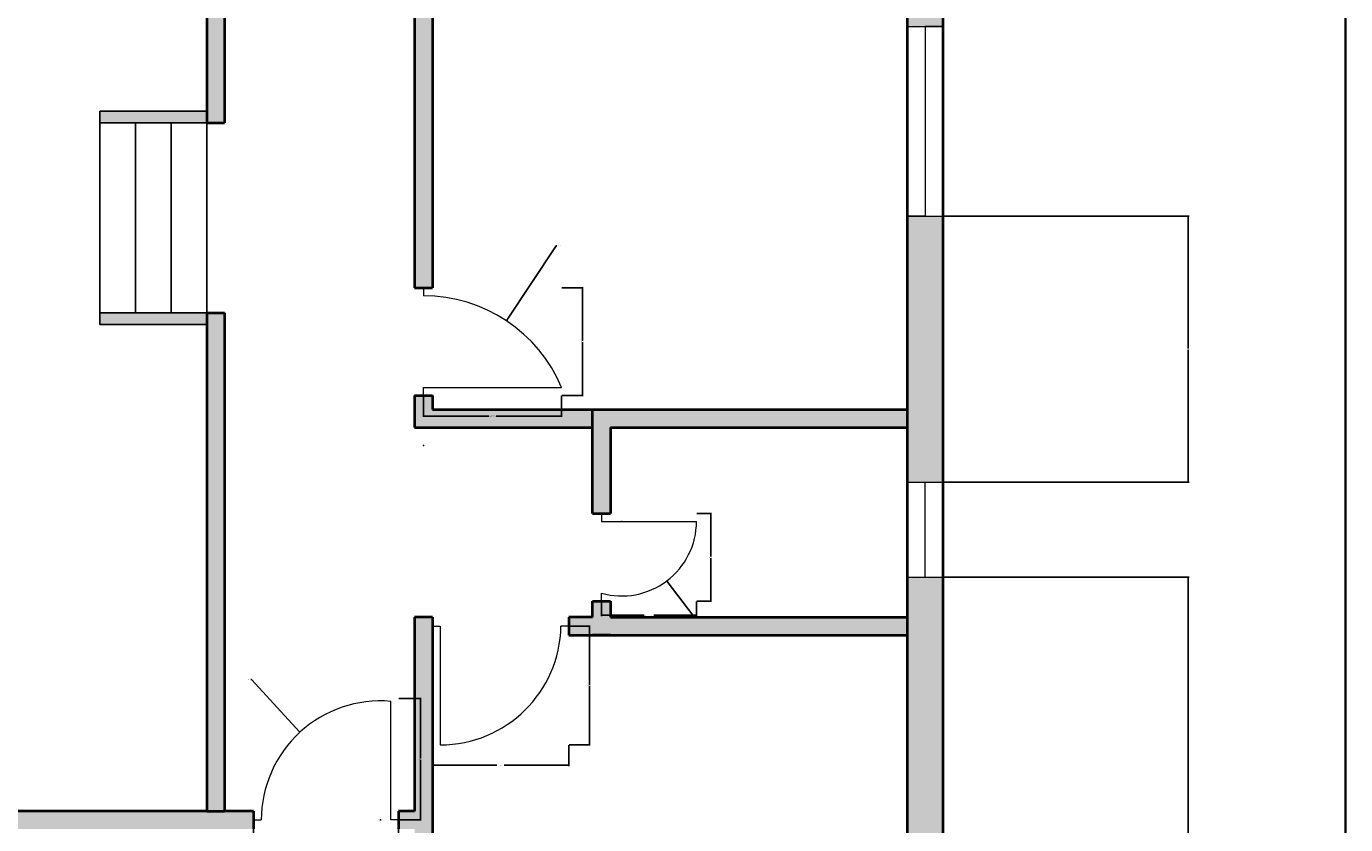
# Model space of a CAD drawing. Units: inches. Extents: x 1441 to 2460, y 1648 to 2683.
# Tile 32 of 35: x 2127 to 2460, y 1922 to 2124. Entities that reach past the tile are written whole.
import ezdxf

# ---------------------------------------------------------------- set-up
doc = ezdxf.new("R2010")
doc.units = ezdxf.units.IN
for name, color, linetype, lineweight in [('A-ANNO-DIMS', 2, 'Continuous', 18), ('A-ANNO-TTLB', 7, 'Continuous', 35), ('A-DOOR', 3, 'Continuous', 20), ('A-FLOR-STRS', 7, 'Continuous', 25), ('A-GLAZ', 4, 'Continuous', 18), ('A-WALL', 7, 'Continuous', 40)]:
    doc.layers.add(name, color=color, linetype=linetype, lineweight=lineweight)
doc.layers.add('A-WALL-PATT', color=251, linetype='Continuous', lineweight=13, true_color=0x636466)
doc.styles.get("Standard").update_dxf_attribs({"font": 'arial.ttf'})
doc.dimstyles.get("Standard").update_dxf_attribs({"dimtxt": 0.18, "dimasz": 0.18, "dimexe": 0.18, "dimexo": 0.0625, "dimgap": 0.09, "dimtad": 0, "dimtih": 1, "dimtoh": 1, "dimdec": 4, "dimzin": 0, "dimdsep": 46, "dimtxsty": 'Standard', "dimcen": 0.09, "dimadec": 0, "dimazin": 0, "dimtfac": 1, "dimtdec": 4, "dimtofl": 0, "dimtmove": 0, "dimatfit": 3, "dimfxl": 1, "dimtolj": 1, "dimtzin": 0, "dimarcsym": 0})

# ---------------------------------------------------------------- blocks, each defined once
blk = doc.blocks.new('DOOR-BED2-30')
for p, q in [((0, 27.22), (0, 25.22)), ((0, 0), (0, 2)), ((0, 2), (4.91, 2)), ((4.91, 2), (34.91, 2))]:
    blk.add_line(p, q)
blk.add_arc((0, -12.65), 37.87, 22.7676, 90)
blk = doc.blocks.new('DOOR-WC-SOUTH-24')
for p, q in [((0, 22.15), (0, 20.15)), ((0, 20.15), (24, 20.15)), ((0, 0), (0, 2))]:
    blk.add_line(p, q)
blk.add_arc((5.13, 20.15), 18.86, 254.1904, 0)
blk = doc.blocks.new('DOOR-BED3-30')
for p, q in [((0, 30.01), (2, 30.01)), ((2, 30.01), (2, 0.01)), ((34.49, 30.01), (32.49, 30.01))]:
    blk.add_line(p, q)
blk.add_arc((2, 30.51), 30.5, 270, 359.0598)
blk = doc.blocks.new('DOOR-ENTRY-INNER')
for p, q in [((34.71, 24.01), (34.71, 30.01)), ((34.71, 0.01), (34.71, 24.01)), ((0, 0.01), (2, 0.01)), ((36.71, 0.01), (34.71, 0.01))]:
    blk.add_line(p, q)
blk.add_arc((32.11, 0.01), 30.11, 85.0485, 180)
blk = doc.blocks.new('WIN-48-SASH')
for p, q in [((9, 48), (4.5, 48)), ((4.5, 48), (4.5, 0)), ((4.5, 0), (0, 0))]:
    blk.add_line(p, q)
blk = doc.blocks.new('WIN-24-SASH')
for p, q in [((9, 24), (4.5, 24)), ((4.5, 24), (4.5, 0)), ((4.5, 0), (0, 0))]:
    blk.add_line(p, q)
blk = doc.blocks.new('*D48')
at = {"layer": 'A-ANNO-DIMS', "color": 0, "lineweight": -2, "transparency": 16777216}
for p, q in [((2227.15, 2030.73), (2227.15, 2025.37)), ((2262.07, 2030.73), (2262.07, 2025.37)), ((2227.33, 2025.55), (2243.68, 2025.55)), ((2261.89, 2025.55), (2245.54, 2025.55))]:
    blk.add_line(p, q, dxfattribs=at)
at = {"layer": 'A-ANNO-DIMS', "color": 0, "transparency": 16777216}
for points in [[(2227.33, 2025.58), (2227.33, 2025.52), (2227.15, 2025.55)], [(2261.89, 2025.58), (2261.89, 2025.52), (2262.07, 2025.55)]]:
    blk.add_solid(points, dxfattribs=at)
at = {"layer": 'Defpoints', "color": 0, "transparency": 16777216}
for p in [(2227.15, 2030.79), (2262.07, 2030.79), (2262.07, 2025.55)]:
    blk.add_point(p, dxfattribs=at)
at = {"layer": 'A-ANNO-DIMS', "color": 0, "transparency": 16777216, "insert": (2244.61, 2025.55), "char_height": 0.18, "attachment_point": 5}
blk.add_mtext('\\A1;B2 DR 35 TYP.', dxfattribs=at)
blk = doc.blocks.new('*D49')
at = {"layer": 'A-ANNO-DIMS', "color": 0, "lineweight": -2, "transparency": 16777216}
for p, q in [((2262.13, 2058.01), (2267.49, 2058.01)), ((2267.31, 2057.83), (2267.31, 2044.58)), ((2267.31, 2030.97), (2267.31, 2044.22)), ((2262.13, 2030.79), (2267.49, 2030.79))]:
    blk.add_line(p, q, dxfattribs=at)
at = {"layer": 'A-ANNO-DIMS', "color": 0, "transparency": 16777216}
for points in [[(2267.28, 2057.83), (2267.34, 2057.83), (2267.31, 2058.01)], [(2267.28, 2030.97), (2267.34, 2030.97), (2267.31, 2030.79)]]:
    blk.add_solid(points, dxfattribs=at)
at = {"layer": 'Defpoints', "color": 0, "transparency": 16777216}
for p in [(2262.07, 2058.01), (2267.31, 2058.01), (2262.07, 2030.79)]:
    blk.add_point(p, dxfattribs=at)
at = {"layer": 'A-ANNO-DIMS', "color": 0, "transparency": 16777216, "insert": (2267.31, 2044.4), "char_height": 0.18, "attachment_point": 5}
blk.add_mtext('\\A1;27 TYP.', dxfattribs=at)
blk = doc.blocks.new('*D50')
at = {"layer": 'A-ANNO-DIMS', "color": 0, "lineweight": -2, "transparency": 16777216}
for p, q in [((2272.15, 1978.73), (2272.15, 1975.02)), ((2296.15, 1978.73), (2296.15, 1975.02)), ((2272.33, 1975.2), (2282.96, 1975.2)), ((2295.97, 1975.2), (2285.34, 1975.2))]:
    blk.add_line(p, q, dxfattribs=at)
at = {"layer": 'A-ANNO-DIMS', "color": 0, "transparency": 16777216}
for points in [[(2272.33, 1975.23), (2272.33, 1975.17), (2272.15, 1975.2)], [(2295.97, 1975.23), (2295.97, 1975.17), (2296.15, 1975.2)]]:
    blk.add_solid(points, dxfattribs=at)
at = {"layer": 'Defpoints', "color": 0, "transparency": 16777216}
for p in [(2272.15, 1978.8), (2296.15, 1978.8), (2296.15, 1975.2)]:
    blk.add_point(p, dxfattribs=at)
at = {"layer": 'A-ANNO-DIMS', "color": 0, "transparency": 16777216, "insert": (2284.15, 1975.2), "char_height": 0.18, "attachment_point": 5}
blk.add_mtext('\\A1;WC DOOR 24 TYP.', dxfattribs=at)
blk = doc.blocks.new('*D51')
at = {"layer": 'A-ANNO-DIMS', "color": 0, "lineweight": -2, "transparency": 16777216}
for p, q in [((2296.21, 2000.95), (2299.93, 2000.95)), ((2299.75, 2000.77), (2299.75, 1990.05)), ((2299.75, 1978.98), (2299.75, 1989.69)), ((2296.21, 1978.8), (2299.93, 1978.8))]:
    blk.add_line(p, q, dxfattribs=at)
at = {"layer": 'A-ANNO-DIMS', "color": 0, "transparency": 16777216}
for points in [[(2299.72, 2000.77), (2299.78, 2000.77), (2299.75, 2000.95)], [(2299.72, 1978.98), (2299.78, 1978.98), (2299.75, 1978.8)]]:
    blk.add_solid(points, dxfattribs=at)
at = {"layer": 'Defpoints', "color": 0, "transparency": 16777216}
for p in [(2296.15, 2000.95), (2299.75, 2000.95), (2296.15, 1978.8)]:
    blk.add_point(p, dxfattribs=at)
at = {"layer": 'A-ANNO-DIMS', "color": 0, "transparency": 16777216, "insert": (2299.75, 1989.87), "char_height": 0.18, "attachment_point": 5}
blk.add_mtext('\\A1;22 TYP.', dxfattribs=at)
blk = doc.blocks.new('*D52')
at = {"layer": 'A-ANNO-DIMS', "color": 0, "lineweight": -2, "transparency": 16777216}
for p, q in [((2229.4, 1942.38), (2229.4, 1937.09)), ((2263.9, 1942.38), (2263.9, 1937.09)), ((2229.58, 1937.27), (2245.72, 1937.27)), ((2263.72, 1937.27), (2247.58, 1937.27))]:
    blk.add_line(p, q, dxfattribs=at)
at = {"layer": 'A-ANNO-DIMS', "color": 0, "transparency": 16777216}
for points in [[(2229.58, 1937.3), (2229.58, 1937.24), (2229.4, 1937.27)], [(2263.72, 1937.3), (2263.72, 1937.24), (2263.9, 1937.27)]]:
    blk.add_solid(points, dxfattribs=at)
at = {"layer": 'Defpoints', "color": 0, "transparency": 16777216}
for p in [(2229.4, 1942.45), (2263.9, 1942.45), (2263.9, 1937.27)]:
    blk.add_point(p, dxfattribs=at)
at = {"layer": 'A-ANNO-DIMS', "color": 0, "transparency": 16777216, "insert": (2246.65, 1937.27), "char_height": 0.18, "attachment_point": 5}
blk.add_mtext('\\A1;B3 DR 34 TYP.', dxfattribs=at)
blk = doc.blocks.new('*D53')
at = {"layer": 'A-ANNO-DIMS', "color": 0, "lineweight": -2, "transparency": 16777216}
for p, q in [((2263.96, 1972.45), (2269.25, 1972.45)), ((2269.07, 1972.27), (2269.07, 1957.63)), ((2269.07, 1942.63), (2269.07, 1957.26)), ((2263.96, 1942.45), (2269.25, 1942.45))]:
    blk.add_line(p, q, dxfattribs=at)
at = {"layer": 'A-ANNO-DIMS', "color": 0, "transparency": 16777216}
for points in [[(2269.04, 1972.27), (2269.1, 1972.27), (2269.07, 1972.45)], [(2269.04, 1942.63), (2269.1, 1942.63), (2269.07, 1942.45)]]:
    blk.add_solid(points, dxfattribs=at)
at = {"layer": 'Defpoints', "color": 0, "transparency": 16777216}
for p in [(2263.9, 1972.45), (2269.07, 1972.45), (2263.9, 1942.45)]:
    blk.add_point(p, dxfattribs=at)
at = {"layer": 'A-ANNO-DIMS', "color": 0, "transparency": 16777216, "insert": (2269.07, 1957.45), "char_height": 0.18, "attachment_point": 5}
blk.add_mtext('\\A1;30 TYP.', dxfattribs=at)
blk = doc.blocks.new('*D56')
at = {"layer": 'A-ANNO-DIMS', "color": 0, "lineweight": -2, "transparency": 16777216}
for p, q in [((2184.17, 1923.38), (2184.17, 1917.76)), ((2220.88, 1923.38), (2220.88, 1917.76)), ((2184.35, 1917.94), (2201.59, 1917.94)), ((2220.7, 1917.94), (2203.46, 1917.94))]:
    blk.add_line(p, q, dxfattribs=at)
at = {"layer": 'A-ANNO-DIMS', "color": 0, "transparency": 16777216}
for points in [[(2184.35, 1917.97), (2184.35, 1917.91), (2184.17, 1917.94)], [(2220.7, 1917.97), (2220.7, 1917.91), (2220.88, 1917.94)]]:
    blk.add_solid(points, dxfattribs=at)
at = {"layer": 'Defpoints', "color": 0, "transparency": 16777216}
for p in [(2184.17, 1923.45), (2220.88, 1923.45), (2220.88, 1917.94)]:
    blk.add_point(p, dxfattribs=at)
at = {"layer": 'A-ANNO-DIMS', "color": 0, "transparency": 16777216, "insert": (2202.52, 1917.94), "char_height": 0.18, "attachment_point": 5}
blk.add_mtext('\\A1;DOOR 37 TYP.', dxfattribs=at)
blk = doc.blocks.new('*D57')
at = {"layer": 'A-ANNO-DIMS', "color": 0, "lineweight": -2, "transparency": 16777216}
for p, q in [((2220.94, 1954.17), (2226.56, 1954.17)), ((2226.38, 1953.99), (2226.38, 1938.99)), ((2226.38, 1923.63), (2226.38, 1938.63)), ((2220.94, 1923.45), (2226.56, 1923.45))]:
    blk.add_line(p, q, dxfattribs=at)
at = {"layer": 'A-ANNO-DIMS', "color": 0, "transparency": 16777216}
for points in [[(2226.35, 1953.99), (2226.41, 1953.99), (2226.38, 1954.17)], [(2226.35, 1923.63), (2226.41, 1923.63), (2226.38, 1923.45)]]:
    blk.add_solid(points, dxfattribs=at)
at = {"layer": 'Defpoints', "color": 0, "transparency": 16777216}
for p in [(2220.88, 1954.17), (2226.38, 1954.17), (2220.88, 1923.45)]:
    blk.add_point(p, dxfattribs=at)
at = {"layer": 'A-ANNO-DIMS', "color": 0, "transparency": 16777216, "insert": (2226.38, 1938.81), "char_height": 0.18, "attachment_point": 5}
blk.add_mtext('\\A1;31 TYP.', dxfattribs=at)
blk = doc.blocks.new('*D81')
at = {"layer": 'A-ANNO-DIMS', "color": 0, "lineweight": -2, "transparency": 16777216}
for p, q in [((2037.84, 2298.7), (1976.42, 2298.7)), ((1976.6, 2298.52), (1976.6, 2055.94)), ((1976.6, 1813), (1976.6, 2055.57)), ((2154.24, 1812.82), (1976.42, 1812.82))]:
    blk.add_line(p, q, dxfattribs=at)
at = {"layer": 'A-ANNO-DIMS', "color": 0, "transparency": 16777216}
for points in [[(1976.57, 2298.52), (1976.63, 2298.52), (1976.6, 2298.7)], [(1976.57, 1813), (1976.63, 1813), (1976.6, 1812.82)]]:
    blk.add_solid(points, dxfattribs=at)
at = {"layer": 'Defpoints', "color": 0, "transparency": 16777216}
for p in [(1976.6, 2298.7), (2037.9, 2298.7), (2154.3, 1812.82)]:
    blk.add_point(p, dxfattribs=at)
at = {"layer": 'A-ANNO-DIMS', "color": 0, "transparency": 16777216, "insert": (1976.6, 2055.76), "char_height": 0.18, "attachment_point": 5}
blk.add_mtext('\\A1;485.9', dxfattribs=at)
blk = doc.blocks.new('*D86')
at = {"layer": 'A-ANNO-DIMS', "color": 0, "lineweight": -2, "transparency": 16777216}
for p, q in [((2358.46, 1984.83), (2420.62, 1984.83)), ((2420.44, 1984.65), (2420.44, 1909.69)), ((2420.44, 1834.38), (2420.44, 1909.33)), ((2358.46, 1834.2), (2420.62, 1834.2))]:
    blk.add_line(p, q, dxfattribs=at)
at = {"layer": 'A-ANNO-DIMS', "color": 0, "transparency": 16777216}
for points in [[(2420.41, 1984.65), (2420.47, 1984.65), (2420.44, 1984.83)], [(2420.41, 1834.38), (2420.47, 1834.38), (2420.44, 1834.2)]]:
    blk.add_solid(points, dxfattribs=at)
at = {"layer": 'Defpoints', "color": 0, "transparency": 16777216}
for p in [(2358.4, 1984.83), (2420.44, 1984.83), (2358.4, 1834.2)]:
    blk.add_point(p, dxfattribs=at)
at = {"layer": 'A-ANNO-DIMS', "color": 0, "transparency": 16777216, "insert": (2420.44, 1909.51), "char_height": 0.18, "attachment_point": 5}
blk.add_mtext('\\A1;150.64', dxfattribs=at)
blk = doc.blocks.new('*D87')
at = {"layer": 'A-ANNO-DIMS', "color": 0, "lineweight": -2, "transparency": 16777216}
for p, q in [((2358.46, 2076.11), (2420.62, 2076.11)), ((2420.44, 2075.93), (2420.44, 2042.65)), ((2420.44, 2009.01), (2420.44, 2042.29)), ((2358.46, 2008.83), (2420.62, 2008.83))]:
    blk.add_line(p, q, dxfattribs=at)
at = {"layer": 'A-ANNO-DIMS', "color": 0, "transparency": 16777216}
for points in [[(2420.41, 2075.93), (2420.47, 2075.93), (2420.44, 2076.11)], [(2420.41, 2009.01), (2420.47, 2009.01), (2420.44, 2008.83)]]:
    blk.add_solid(points, dxfattribs=at)
at = {"layer": 'Defpoints', "color": 0, "transparency": 16777216}
for p in [(2358.4, 2076.11), (2420.44, 2076.11), (2358.4, 2008.83)]:
    blk.add_point(p, dxfattribs=at)
at = {"layer": 'A-ANNO-DIMS', "color": 0, "transparency": 16777216, "insert": (2420.44, 2042.47), "char_height": 0.18, "attachment_point": 5}
blk.add_mtext('\\A1;67.28', dxfattribs=at)
blk = doc.blocks.new('*D129')
at = {"layer": 'A-ANNO-DIMS', "color": 0, "lineweight": -2, "transparency": 16777216}
for p, q in [((2260.7, 2068.59), (2248.22, 2049.82)), ((2260.88, 2068.59), (2260.7, 2068.59)), ((2227.06, 2018.14), (2227.24, 2018.14)), ((2227.15, 2018.05), (2227.15, 2018.23))]:
    blk.add_line(p, q, dxfattribs=at)
at = {"layer": 'A-ANNO-DIMS', "color": 0, "transparency": 16777216}
blk.add_solid([(2248.19, 2049.84), (2248.24, 2049.81), (2248.12, 2049.67)], dxfattribs=at)
at = {"layer": 'Defpoints', "color": 0, "transparency": 16777216}
for p in [(2248.12, 2049.67), (2227.15, 2018.14)]:
    blk.add_point(p, dxfattribs=at)
at = {"layer": 'A-ANNO-DIMS', "color": 0, "transparency": 16777216, "insert": (2261.36, 2068.59), "char_height": 0.18, "attachment_point": 5}
blk.add_mtext('\\A1;R37.87', dxfattribs=at)
blk = doc.blocks.new('*D132')
at = {"layer": 'A-ANNO-DIMS', "color": 0, "lineweight": -2, "transparency": 16777216}
for p, q in [((2183.53, 1958.95), (2183.71, 1958.95)), ((2183.71, 1958.95), (2195.8, 1945.77)), ((2216.19, 1923.45), (2216.37, 1923.45)), ((2216.28, 1923.36), (2216.28, 1923.54))]:
    blk.add_line(p, q, dxfattribs=at)
at = {"layer": 'A-ANNO-DIMS', "color": 0, "transparency": 16777216}
blk.add_solid([(2195.83, 1945.79), (2195.78, 1945.75), (2195.93, 1945.64)], dxfattribs=at)
at = {"layer": 'Defpoints', "color": 0, "transparency": 16777216}
for p in [(2195.93, 1945.64), (2216.28, 1923.45)]:
    blk.add_point(p, dxfattribs=at)
at = {"layer": 'A-ANNO-DIMS', "color": 0, "transparency": 16777216, "insert": (2183.07, 1958.95), "char_height": 0.18, "attachment_point": 5}
blk.add_mtext('\\A1;R30.11', dxfattribs=at)
blk = doc.blocks.new('*D135')
at = {"layer": 'A-ANNO-DIMS', "color": 0, "lineweight": -2, "transparency": 16777216}
for p, q in [((2277.2, 1998.95), (2277.38, 1998.95)), ((2277.29, 1998.86), (2277.29, 1999.04)), ((2295.49, 1974.87), (2288.77, 1983.76)), ((2295.67, 1974.87), (2295.49, 1974.87))]:
    blk.add_line(p, q, dxfattribs=at)
at = {"layer": 'A-ANNO-DIMS', "color": 0, "transparency": 16777216}
blk.add_solid([(2288.8, 1983.78), (2288.75, 1983.74), (2288.67, 1983.9)], dxfattribs=at)
at = {"layer": 'Defpoints', "color": 0, "transparency": 16777216}
for p in [(2277.29, 1998.95), (2288.67, 1983.9)]:
    blk.add_point(p, dxfattribs=at)
at = {"layer": 'A-ANNO-DIMS', "color": 0, "transparency": 16777216, "insert": (2296.15, 1974.87), "char_height": 0.18, "attachment_point": 5}
blk.add_mtext('\\A1;R18.86', dxfattribs=at)

msp = doc.modelspace()

# ---------------------------------------------------------------- hatches: boundary and pattern name
at = {"layer": 'A-WALL-PATT'}
h = msp.add_hatch(color=256, dxfattribs=at)
h.dxf.hatch_style = 1
h.paths.add_polyline_path([(2096.524, 2298.6952), (2037.9015, 2298.6952), (2037.9015, 2246.9605), (2046.9015, 2246.9605), (2046.9015, 2289.6952), (2096.524, 2289.6952), (2096.524, 2294.1952)])
h.paths.add_polyline_path([(2144.5933, 2298.6952), (2120.524, 2298.6952), (2120.524, 2289.6952), (2144.5933, 2289.6952), (2144.5933, 2294.1952)])
h.paths.add_polyline_path([(2136.4015, 2289.6952), (2131.9015, 2289.6952), (2131.9015, 2233.0622), (2136.4015, 2233.0622)])
h.paths.add_polyline_path([(2184.8877, 2294.3362), (2184.8877, 2295.2788), (2184.8877, 2298.6952), (2168.5933, 2298.6952), (2168.5933, 2289.6952), (2184.8877, 2289.6952)])
h.paths.add_polyline_path([(2176.9015, 2289.6952), (2172.4015, 2289.6952), (2172.4015, 2199.6952), (2176.9015, 2199.6952)])
h.paths.add_polyline_path([(2229.4015, 2204.637), (2224.9015, 2204.637), (2224.9015, 2199.6952), (2136.4015, 2199.6952), (2136.4015, 2204.637), (2131.9015, 2204.637), (2131.9015, 2195.1952), (2229.4015, 2195.1952)])
h.paths.add_polyline_path([(2229.4015, 2289.6952), (2224.9015, 2289.6952), (2224.9015, 2233.0622), (2229.4015, 2233.0622)])
h.paths.add_polyline_path([(2358.4015, 2298.6952), (2208.8877, 2298.6952), (2208.8877, 2289.6952), (2349.4015, 2289.6952), (2349.4015, 2250.8051), (2358.4015, 2250.8051)])
h.paths.add_polyline_path([(2358.4015, 2202.8051), (2349.4015, 2202.8051), (2349.4015, 2157.6952), (2216.9636, 2157.6952), (2216.9636, 2153.1952), (2224.9015, 2153.1952), (2224.9015, 2058.005), (2229.4015, 2058.005), (2229.4015, 2153.1952), (2349.4015, 2153.1952), (2349.4015, 2124.108), (2358.4015, 2124.108)])
h.paths.add_polyline_path([(2358.4015, 1984.8305), (2349.4015, 1984.8305), (2349.4015, 1834.1952), (2358.4015, 1834.1952)])
h.paths.add_polyline_path([(2358.4015, 2076.108), (2349.4015, 2076.108), (2349.4015, 2008.8305), (2358.4015, 2008.8305)])
h.paths.add_polyline_path([(2349.4015, 2027.1952), (2269.9015, 2027.1952), (2269.9015, 2000.9452), (2274.4015, 2000.9452), (2274.4015, 2022.6952), (2349.4015, 2022.6952)])
h.paths.add_polyline_path([(2269.9015, 2027.1952), (2229.4015, 2027.1952), (2229.4015, 2030.7912), (2224.9015, 2030.7912), (2224.9015, 2022.6952), (2269.9015, 2022.6952)])
h.paths.add_polyline_path([(2349.4015, 1974.6952), (2274.4015, 1974.6952), (2274.4015, 1978.7973), (2269.9015, 1978.7973), (2269.9015, 1974.6952), (2263.8979, 1974.6952), (2263.8979, 1970.1952), (2269.9015, 1970.1952), (2274.4015, 1970.1952), (2349.4015, 1970.1952)])
h.paths.add_polyline_path([(2229.4015, 1974.6952), (2224.9015, 1974.6952), (2224.9015, 1925.6952), (2220.8772, 1925.6952), (2220.8772, 1921.1952), (2229.4015, 1921.1952)])
h.paths.add_polyline_path([(2229.4015, 1921.1952), (2224.9015, 1921.1952), (2224.9015, 1843.1952), (2229.4015, 1843.1952)])
h.paths.add_polyline_path([(2268.1291, 1838.6952), (2268.1291, 1843.1952), (2229.4015, 1843.1952), (2220.91, 1843.1952), (2220.91, 1834.1952), (2227.1771, 1834.1952), (2268.1291, 1834.1952)])
h.paths.add_polyline_path([(2349.4015, 1843.1952), (2328.1291, 1843.1952), (2328.1291, 1834.1952), (2349.4015, 1834.1952)])
h.paths.add_polyline_path([(2046.9015, 1857.7914), (2037.9015, 1857.7914), (2037.9015, 1834.1952), (2164.019, 1834.1952), (2164.019, 1838.6952), (2164.019, 1843.1952), (2046.9015, 1843.1952)])
h.paths.add_polyline_path([(2046.9015, 1959.2399), (2042.4015, 1959.2399), (2037.9015, 1959.2399), (2037.9015, 1905.7914), (2046.9015, 1905.7914), (2046.9015, 1921.1952), (2172.4015, 1921.1952), (2176.9015, 1921.1952), (2184.1657, 1921.1952), (2184.1657, 1925.6952), (2176.9015, 1925.6952), (2172.4015, 1925.6952), (2046.9015, 1925.6952)])
h.paths.add_polyline_path([(2046.9015, 2106.6907), (2037.9015, 2106.6907), (2037.9015, 2019.2399), (2046.9015, 2019.2399)])
h.paths.add_polyline_path([(2176.9015, 2051.6952), (2172.4015, 2051.6952), (2172.4015, 2048.6952), (2172.4015, 1925.6952), (2176.9015, 1925.6952)])
h.paths.add_polyline_path([(2172.4015, 2051.6952), (2145.4015, 2051.6952), (2145.4015, 2048.6952), (2172.4015, 2048.6952)])
h.paths.add_polyline_path([(2172.4015, 2102.6952), (2145.4015, 2102.6952), (2145.4015, 2099.6952), (2154.4015, 2099.6952), (2172.4015, 2099.6952)])
h.paths.add_polyline_path([(2176.9015, 2153.1952), (2179.5767, 2153.1952), (2179.5767, 2157.6952), (2176.9015, 2157.6952), (2176.9015, 2195.1952), (2172.4015, 2195.1952), (2172.4015, 2099.6952), (2176.9015, 2099.6952)])
h.paths.add_polyline_path([(2046.9015, 2198.9605), (2037.9015, 2198.9605), (2037.9015, 2166.6907), (2046.9015, 2166.6907)])

# ---------------------------------------------------------------- linework, layer by layer
at = {"layer": 'A-ANNO-TTLB'}
msp.add_lwpolyline([(1440.5107, 2682.6413), (2460.193, 2682.6413), (2460.193, 1648.08), (1440.5107, 1648.08)], close=True, dxfattribs=at)
at = {"layer": 'A-FLOR-STRS'}
for p, q in [((2172.4015, 2102.6952), (2145.4015, 2102.6952)), ((2145.4015, 2048.6952), (2145.4015, 2102.6952)), ((2172.4015, 2099.6952), (2172.4015, 2102.6952)), ((2172.4015, 2102.6952), (2172.4015, 2099.6952)), ((2172.4015, 2099.6952), (2145.4015, 2099.6952)), ((2154.4015, 2099.6952), (2145.4015, 2099.6952)), ((2145.4015, 2099.6952), (2145.4015, 2048.6952)), ((2154.4015, 2051.6952), (2154.4015, 2099.6952)), ((2172.4015, 2099.6952), (2163.4015, 2099.6952)), ((2163.4015, 2099.6952), (2163.4015, 2051.6952)), ((2172.4015, 2051.6952), (2172.4015, 2099.6952)), ((2172.4015, 2051.6952), (2145.4015, 2051.6952)), ((2163.4015, 2051.6952), (2154.4015, 2051.6952)), ((2172.4015, 2048.6952), (2172.4015, 2051.6952)), ((2172.4015, 2048.6952), (2172.4015, 2051.6952)), ((2172.4015, 2048.6952), (2145.4015, 2048.6952))]:
    msp.add_line(p, q, dxfattribs=at)
at = {"layer": 'A-GLAZ'}
for p, q in [((2349.4015, 2124.108), (2358.4015, 2124.108)), ((2349.4015, 2076.108), (2358.4015, 2076.108)), ((2349.4015, 2008.8305), (2358.4015, 2008.8305)), ((2349.4015, 1984.8305), (2358.4015, 1984.8305))]:
    msp.add_line(p, q, dxfattribs=at)
at = {"layer": 'A-WALL'}
for p, q in [((2358.4015, 2298.6952), (2358.4015, 1834.1952)), ((2172.4015, 2195.1952), (2172.4015, 2099.6952)), ((2176.9015, 2153.1952), (2176.9015, 2099.6952)), ((2224.9015, 2153.1952), (2224.9015, 2058.005)), ((2229.4015, 2153.1952), (2229.4015, 2058.005)), ((2349.4015, 2153.1952), (2349.4015, 1834.1952)), ((2172.4015, 2099.6952), (2176.9015, 2099.6952)), ((2224.9015, 2058.005), (2229.4015, 2058.005)), ((2172.4015, 2051.6952), (2172.4015, 1925.6952)), ((2172.4015, 2051.6952), (2176.9015, 2051.6952)), ((2176.9015, 2051.6952), (2176.9015, 1925.6952)), ((2224.9015, 2030.7912), (2224.9015, 2022.6952)), ((2224.9015, 2030.7912), (2229.4015, 2030.7912)), ((2229.4015, 2030.7912), (2229.4015, 2027.1952)), ((2229.4015, 2027.1952), (2349.4015, 2027.1952)), ((2269.9015, 2000.9452), (2269.9015, 2027.1952)), ((2224.9015, 2022.6952), (2269.9015, 2022.6952)), ((2274.4015, 2022.6952), (2274.4015, 2000.9452)), ((2274.4015, 2022.6952), (2349.4015, 2022.6952)), ((2269.9015, 2000.9452), (2274.4015, 2000.9452)), ((2269.9015, 1974.6952), (2269.9015, 1978.7973)), ((2269.9015, 1978.7973), (2269.9015, 1978.7973)), ((2269.9015, 1978.7973), (2274.4015, 1978.7973)), ((2274.4015, 1978.7973), (2274.4015, 1974.6952)), ((2224.9015, 1974.6952), (2224.9015, 1925.6952)), ((2229.4015, 1974.6952), (2224.9015, 1974.6952)), ((2229.4015, 1974.6952), (2229.4015, 1843.1952)), ((2269.9015, 1974.6952), (2263.8979, 1974.6952)), ((2263.8979, 1974.6952), (2263.8979, 1974.6952)), ((2263.8979, 1974.6952), (2263.8979, 1970.1952)), ((2274.4015, 1974.6952), (2349.4015, 1974.6952)), ((2263.8979, 1970.1952), (2269.9015, 1970.1952)), ((2269.9015, 1970.1952), (2349.4015, 1970.1952)), ((2274.4015, 1970.1952), (2269.9015, 1970.1952)), ((2172.4015, 1925.6952), (2046.9015, 1925.6952)), ((2172.4015, 1925.6952), (2176.9015, 1925.6952)), ((2184.1657, 1925.6952), (2176.9015, 1925.6952)), ((2184.1657, 1925.6952), (2184.1657, 1921.1952)), ((2224.9015, 1925.6952), (2220.8772, 1925.6952)), ((2220.8772, 1925.6952), (2220.8772, 1921.1952))]:
    msp.add_line(p, q, dxfattribs=at)

# ---------------------------------------------------------------- block references
at = {"layer": 'A-DOOR'}
for name, p in [('DOOR-BED2-30', (2227.1556, 2030.79)), ('DOOR-WC-SOUTH-24', (2272.1556, 1978.8)), ('DOOR-BED3-30', (2229.4056, 1942.44)), ('DOOR-ENTRY-INNER', (2184.1656, 1923.44))]:
    msp.add_blockref(name, p, dxfattribs=at)
at = {"layer": 'A-GLAZ'}
msp.add_blockref('WIN-48-SASH', (2349.4056, 2076.1074), dxfattribs=at)
at = {"layer": 'A-GLAZ', "rotation": 180}
msp.add_blockref('WIN-24-SASH', (2358.3974, 2008.831), dxfattribs=at)

# ---------------------------------------------------------------- dimensions: what is measured, and where the dimension line sits
at = {"layer": 'A-ANNO-DIMS'}
for base, p1, p2, override, picture, middle in [((1976.6039, 2298.6952), (2154.3041, 1812.8171), (2037.9015, 2298.6952), {"dimdec": 1, "dimlfac": 1, "dimrnd": 0, "dimzin": 0, "dimdsep": 46, "dimlunit": 2}, '*D81', (1976.6039, 2055.7561)), ((2420.439, 2076.108), (2358.4015, 2008.8305), (2358.4015, 2076.108), {"dimdec": 2, "dimlfac": 1, "dimrnd": 0, "dimzin": 0, "dimdsep": 46, "dimlunit": 2}, '*D87', (2420.439, 2042.4692)), ((2420.439, 1984.8305), (2358.4015, 1834.1952), (2358.4015, 1984.8305), {"dimdec": 2, "dimlfac": 1, "dimrnd": 0, "dimzin": 0, "dimdsep": 46, "dimlunit": 2}, '*D86', (2420.439, 1909.5128))]:
    dim = msp.add_linear_dim(base=base, p1=p1, p2=p2, angle=90, dimstyle='Standard', override=override, dxfattribs=at)
    dim.commit()
    dim.dimension.update_dxf_attribs({"geometry": picture, "text_midpoint": middle})
for center, mpoint, picture, middle in [((2227.1515, 2018.1362), (2248.1169, 2049.6719), '*D129', (2261.356, 2068.5933)), ((2277.2901, 1998.9452), (2288.6662, 1983.9007), '*D135', (2296.1516, 1974.874)), ((2216.2781, 1923.4452), (2195.9252, 1945.6378), '*D132', (2183.0709, 1958.9534))]:
    dim = msp.add_radius_dim(center=center, mpoint=mpoint, dimstyle='Standard', override={"dimdec": 2, "dimlfac": 1, "dimrnd": 0, "dimzin": 0, "dimdsep": 46, "dimlunit": 2}, dxfattribs=at)
    dim.commit()
    dim.dimension.update_dxf_attribs({"geometry": picture, "text_midpoint": middle, "dimtype": 164})
for base, p1, p2, picture, middle in [((2267.3074, 2058.005), (2262.0697, 2030.7912), (2262.0697, 2058.005), '*D49', (2267.3074, 2044.3981)), ((2299.7515, 2000.9452), (2296.1515, 1978.7973), (2296.1515, 2000.9452), '*D51', (2299.7515, 1989.8713)), ((2269.0723, 1972.4452), (2263.8979, 1942.4452), (2263.8979, 1972.4452), '*D53', (2269.0723, 1957.4452)), ((2226.3839, 1954.1735), (2220.8772, 1923.4452), (2220.8772, 1954.1735), '*D57', (2226.3839, 1938.8094))]:
    dim = msp.add_linear_dim(base=base, p1=p1, p2=p2, angle=90, text='<> TYP.', dimstyle='Standard', override={"dimdec": 0, "dimlfac": 1, "dimrnd": 0, "dimzin": 0, "dimdsep": 46, "dimlunit": 2}, dxfattribs=at)
    dim.commit()
    dim.dimension.update_dxf_attribs({"geometry": picture, "text_midpoint": middle})
for base, p1, p2, text, picture, middle in [((2262.0697, 2025.5535), (2227.1515, 2030.7912), (2262.0697, 2030.7912), 'B2 DR <> TYP.', '*D48', (2244.6106, 2025.5535)), ((2296.1515, 1975.1973), (2272.1515, 1978.7973), (2296.1515, 1978.7973), 'WC DOOR <> TYP.', '*D50', (2284.1515, 1975.1973)), ((2263.8979, 1937.2707), (2229.4015, 1942.4452), (2263.8979, 1942.4452), 'B3 DR <> TYP.', '*D52', (2246.6497, 1937.2707)), ((2220.8772, 1917.9385), (2184.1657, 1923.4452), (2220.8772, 1923.4452), 'DOOR <> TYP.', '*D56', (2202.5215, 1917.9385))]:
    dim = msp.add_linear_dim(base=base, p1=p1, p2=p2, text=text, dimstyle='Standard', override={"dimdec": 0, "dimlfac": 1, "dimrnd": 0, "dimzin": 0, "dimdsep": 46, "dimlunit": 2}, dxfattribs=at)
    dim.commit()
    dim.dimension.update_dxf_attribs({"geometry": picture, "text_midpoint": middle})

doc.saveas('drawing.dxf')
